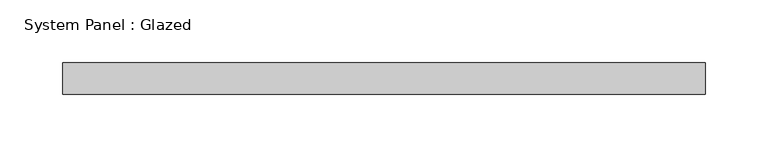
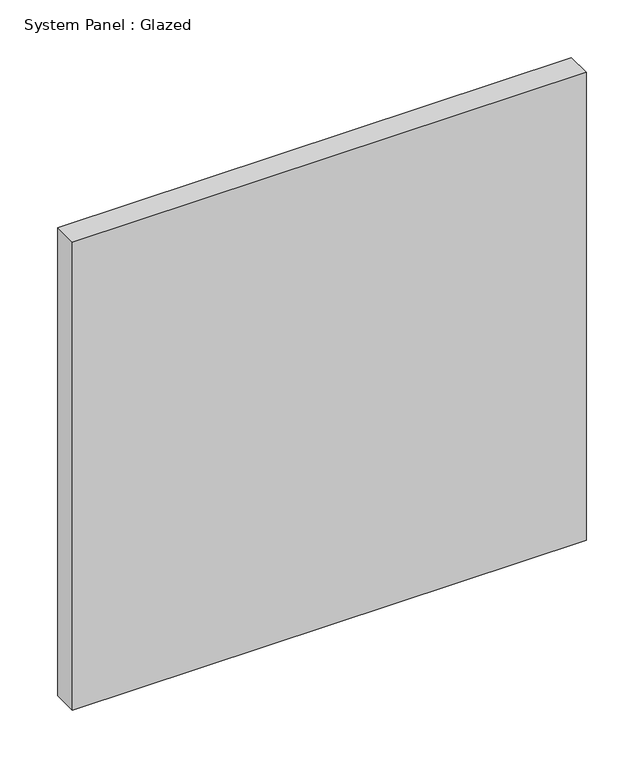
"""IFC4 building model written with IfcOpenShell, lengths in millimetres: plate geometry, System Panel : Glazed."""

from ifc_helpers import new_model, si_unit, origin, origin_with_axes, place, context, project, spatial, polyline, outline, extrude, source, transform, mapped, element, save


def system_panel_glazed_6026b5c4(model_context):
    return source(origin(), model_context, "Body", "SweptSolid", [
        extrude(outline(polyline([(257.175, 19.05), (-257.175, 19.05), (-257.175, 44.45), (257.175, 44.45), (257.175, 19.05)])), origin_with_axes(), (0.0, 0.0, 1.0), 495.3),
    ])


if __name__ == "__main__":
    model = new_model("IFC4")
    model_context = context("Model", 3, world=origin())
    ifc_project = project(units=[si_unit("LENGTHUNIT", "METRE", prefix="MILLI")], contexts=[model_context])
    site = spatial("IfcSite", under=ifc_project)
    building = spatial("IfcBuilding", under=site)
    placement = place(None, origin())
    system_panel_glazed_shape = system_panel_glazed_6026b5c4(model_context)
    element("IfcPlate", 1, ObjectType="System Panel : Glazed", at=placement, inside=building, context=model_context, shape_type="MappedRepresentation", body=[
        mapped(system_panel_glazed_shape, transform((0.0, 0.0, 0.0), x_axis=(1.0, 0.0, 0.0), y_axis=(0.0, 1.0, 0.0), z_axis=(0.0, 0.0, 1.0))),
    ])
    save(model, "model.ifc")

# Revit data of these elements
# Type "System Panel : Glazed"
#   Construction Type Id = "GSP4R"
#   Analytic Construction = "1/8 in Pilkington single glazing"
#   Visual Light Transmittance = 0.9
#   Solar Heat Gain Coefficient = 0.86
#   Heat Transfer Coefficient (U) = 1.18115 BTU/(h·ft²·°F)
#   Define Thermal Properties by = 1
# Element 1 (IfcPlate, "System Panel : Glazed")
#   Materials on its faces: "Glass"
# Materials
#   "Glass": class "Glass", colour RGB 0 128 192, transparency 0.75, Description = "Soda Lime Glass", Cost = 0
